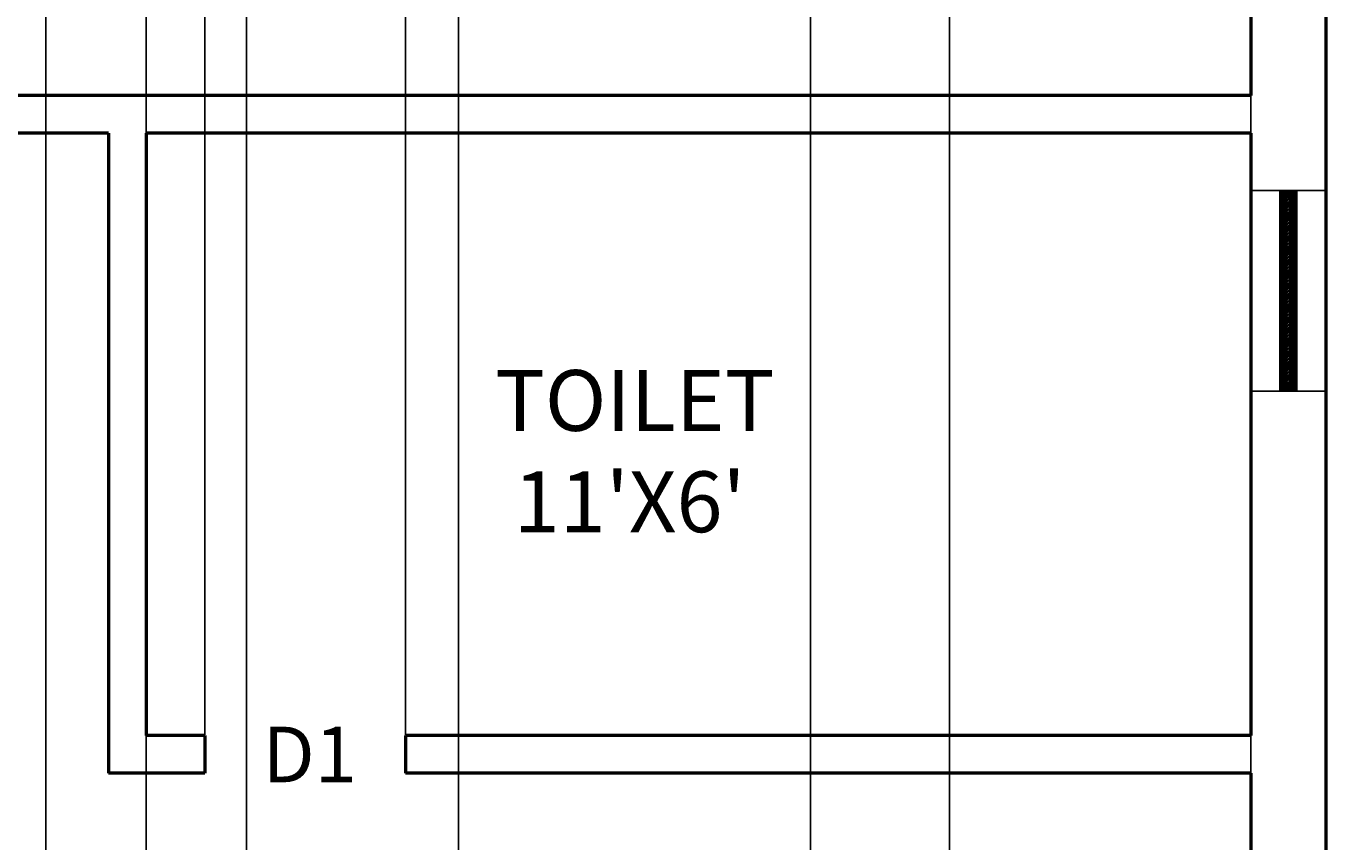
# Model space of a CAD drawing. Units: inches. Extents: x 338 to 1188, y -996 to 127.
# Tile 12 of 15: x 802 to 957, y -483 to -385. Entities that reach past the tile are written whole.
import ezdxf

# ---------------------------------------------------------------- set-up
doc = ezdxf.new("R2010")
doc.units = ezdxf.units.IN
doc.header["$MEASUREMENT"] = 0
for name, color, linetype, lineweight in [('A-ANNO-DIMS', 5, 'Continuous', 18), ('A-ANNO-TEXT', 7, 'Continuous', 18), ('A-AREA-IDEN', 8, 'Continuous', 18), ('A-GLAZ-PATT', 5, 'Continuous', 13), ('wall', 1, 'Continuous', 50), ('win', 5, 'Continuous', 25)]:
    doc.layers.add(name, color=color, linetype=linetype, lineweight=lineweight)
doc.styles.get("Standard").update_dxf_attribs({"font": 'arial.ttf'})
doc.dimstyles.get("Standard").update_dxf_attribs({"dimtxt": 0.18, "dimasz": 0.18, "dimexe": 0.18, "dimexo": 0.0625, "dimgap": 0.09, "dimtad": 0, "dimtih": 1, "dimtoh": 1, "dimdec": 1, "dimzin": 0, "dimdsep": 46, "dimlunit": 4, "dimtxsty": 'Standard', "dimcen": 0.09, "dimadec": 0, "dimazin": 0, "dimtfac": 1, "dimtdec": 1, "dimtofl": 0, "dimtmove": 0, "dimatfit": 3, "dimfxl": 1, "dimtolj": 1, "dimtzin": 0, "dimarcsym": 0})

# ---------------------------------------------------------------- blocks, each defined once
blk = doc.blocks.new('*D26')
at = {"layer": 'A-ANNO-DIMS', "color": 0, "lineweight": -2, "transparency": 16777216}
for p, q in [((815.96, -297.8), (815.96, -968.86)), ((827.96, -297.8), (827.96, -968.86)), ((816.14, -968.68), (821.64, -968.68)), ((827.78, -968.68), (822.28, -968.68))]:
    blk.add_line(p, q, dxfattribs=at)
at = {"layer": 'A-ANNO-DIMS', "color": 0, "transparency": 16777216}
for points in [[(816.14, -968.65), (816.14, -968.71), (815.96, -968.68)], [(827.78, -968.65), (827.78, -968.71), (827.96, -968.68)]]:
    blk.add_solid(points, dxfattribs=at)
at = {"layer": 'Defpoints', "color": 0, "transparency": 16777216}
for p in [(815.96, -297.73), (827.96, -297.73), (827.96, -968.68)]:
    blk.add_point(p, dxfattribs=at)
at = {"layer": 'A-ANNO-DIMS', "color": 0, "transparency": 16777216, "insert": (821.96, -968.68), "char_height": 0.18, "attachment_point": 5}
blk.add_mtext('\\A1;1\'-0"', dxfattribs=at)
blk = doc.blocks.new('*D27')
at = {"layer": 'A-ANNO-DIMS', "color": 0, "lineweight": -2, "transparency": 16777216}
for p, q in [((911.96, -297.8), (911.96, -968.86)), ((947.96, -297.8), (947.96, -968.86)), ((912.14, -968.68), (929.63, -968.68)), ((947.78, -968.68), (930.29, -968.68))]:
    blk.add_line(p, q, dxfattribs=at)
at = {"layer": 'A-ANNO-DIMS', "color": 0, "transparency": 16777216}
for points in [[(912.14, -968.65), (912.14, -968.71), (911.96, -968.68)], [(947.78, -968.65), (947.78, -968.71), (947.96, -968.68)]]:
    blk.add_solid(points, dxfattribs=at)
at = {"layer": 'Defpoints', "color": 0, "transparency": 16777216}
for p in [(911.96, -297.73), (947.96, -297.73), (947.96, -968.68)]:
    blk.add_point(p, dxfattribs=at)
at = {"layer": 'A-ANNO-DIMS', "color": 0, "transparency": 16777216, "insert": (929.96, -968.68), "char_height": 0.18, "attachment_point": 5}
blk.add_mtext('\\A1;3\'-0"', dxfattribs=at)
blk = doc.blocks.new('*D28')
at = {"layer": 'A-ANNO-DIMS', "color": 0, "lineweight": -2, "transparency": 16777216}
for p, q in [((803.96, -265.8), (803.96, -968.86)), ((947.96, -297.8), (947.96, -968.86)), ((804.14, -968.68), (875.57, -968.68)), ((947.78, -968.68), (876.35, -968.68))]:
    blk.add_line(p, q, dxfattribs=at)
at = {"layer": 'A-ANNO-DIMS', "color": 0, "transparency": 16777216}
for points in [[(804.14, -968.65), (804.14, -968.71), (803.96, -968.68)], [(947.78, -968.65), (947.78, -968.71), (947.96, -968.68)]]:
    blk.add_solid(points, dxfattribs=at)
at = {"layer": 'Defpoints', "color": 0, "transparency": 16777216}
for p in [(803.96, -265.73), (947.96, -297.73), (947.96, -968.68)]:
    blk.add_point(p, dxfattribs=at)
at = {"layer": 'A-ANNO-DIMS', "color": 0, "transparency": 16777216, "insert": (875.96, -968.68), "char_height": 0.18, "attachment_point": 5}
blk.add_mtext('\\A1;12\'-0"', dxfattribs=at)
blk = doc.blocks.new('*D38')
at = {"layer": 'A-ANNO-DIMS', "color": 0, "lineweight": -2, "transparency": 16777216}
for p, q in [((822.96, -470.17), (822.96, 67.25)), ((823.14, 67.07), (834.63, 67.07)), ((846.78, 67.07), (835.29, 67.07)), ((846.96, -470.17), (846.96, 67.25))]:
    blk.add_line(p, q, dxfattribs=at)
at = {"layer": 'A-ANNO-DIMS', "color": 0, "transparency": 16777216}
for points in [[(823.14, 67.1), (823.14, 67.04), (822.96, 67.07)], [(846.78, 67.1), (846.78, 67.04), (846.96, 67.07)]]:
    blk.add_solid(points, dxfattribs=at)
at = {"layer": 'Defpoints', "color": 0, "transparency": 16777216}
for p in [(846.96, 67.07), (822.96, -470.23), (846.96, -470.23)]:
    blk.add_point(p, dxfattribs=at)
at = {"layer": 'A-ANNO-DIMS', "color": 0, "transparency": 16777216, "insert": (834.96, 67.07), "char_height": 0.18, "attachment_point": 5}
blk.add_mtext('\\A1;2\'-0"', dxfattribs=at)
blk = doc.blocks.new('*D43')
at = {"layer": 'A-ANNO-DIMS', "color": 0, "lineweight": -2, "transparency": 16777216}
for p, q in [((853.28, -53.93), (853.28, -968.86)), ((895.37, -53.93), (895.37, -968.86)), ((853.46, -968.68), (873.99, -968.68)), ((895.19, -968.68), (874.65, -968.68))]:
    blk.add_line(p, q, dxfattribs=at)
at = {"layer": 'A-ANNO-DIMS', "color": 0, "transparency": 16777216}
for points in [[(853.46, -968.65), (853.46, -968.71), (853.28, -968.68)], [(895.19, -968.65), (895.19, -968.71), (895.37, -968.68)]]:
    blk.add_solid(points, dxfattribs=at)
at = {"layer": 'Defpoints', "color": 0, "transparency": 16777216}
for p in [(853.28, -53.87), (895.37, -53.87), (895.37, -968.68)]:
    blk.add_point(p, dxfattribs=at)
at = {"layer": 'A-ANNO-DIMS', "color": 0, "transparency": 16777216, "insert": (874.32, -968.68), "char_height": 0.18, "attachment_point": 5}
blk.add_mtext('\\A1;3\'-6"', dxfattribs=at)
blk = doc.blocks.new('*D44')
at = {"layer": 'A-ANNO-DIMS', "color": 0, "lineweight": -2, "transparency": 16777216}
for p, q in [((895.37, -53.93), (895.37, -968.86)), ((947.96, -54.8), (947.96, -968.86)), ((895.55, -968.68), (921.12, -968.68)), ((947.78, -968.68), (922.21, -968.68))]:
    blk.add_line(p, q, dxfattribs=at)
at = {"layer": 'A-ANNO-DIMS', "color": 0, "transparency": 16777216}
for points in [[(895.55, -968.65), (895.55, -968.71), (895.37, -968.68)], [(947.78, -968.65), (947.78, -968.71), (947.96, -968.68)]]:
    blk.add_solid(points, dxfattribs=at)
at = {"layer": 'Defpoints', "color": 0, "transparency": 16777216}
for p in [(895.37, -53.87), (947.96, -54.73), (947.96, -968.68)]:
    blk.add_point(p, dxfattribs=at)
at = {"layer": 'A-ANNO-DIMS', "color": 0, "transparency": 16777216, "insert": (921.67, -968.68), "char_height": 0.18, "attachment_point": 5}
blk.add_mtext('\\A1;4\'-4 1/2"', dxfattribs=at)
blk = doc.blocks.new('*D47')
at = {"layer": 'A-ANNO-DIMS', "color": 0, "lineweight": -2, "transparency": 16777216}
for p, q in [((759.67, -755.17), (759.67, 67.25)), ((759.85, 67.07), (867.68, 67.07)), ((976.28, 67.07), (868.46, 67.07)), ((976.46, -755.17), (976.46, 67.25))]:
    blk.add_line(p, q, dxfattribs=at)
at = {"layer": 'A-ANNO-DIMS', "color": 0, "transparency": 16777216}
for points in [[(759.85, 67.1), (759.85, 67.04), (759.67, 67.07)], [(976.28, 67.1), (976.28, 67.04), (976.46, 67.07)]]:
    blk.add_solid(points, dxfattribs=at)
at = {"layer": 'Defpoints', "color": 0, "transparency": 16777216}
for p in [(976.46, 67.07), (759.67, -755.23), (976.46, -755.23)]:
    blk.add_point(p, dxfattribs=at)
at = {"layer": 'A-ANNO-DIMS', "color": 0, "transparency": 16777216, "insert": (868.07, 67.07), "char_height": 0.18, "attachment_point": 5}
blk.add_mtext('\\A1;18\'-1"', dxfattribs=at)

msp = doc.modelspace()

# ---------------------------------------------------------------- hatches: boundary and pattern name
at = {"layer": 'A-GLAZ-PATT'}
h = msp.add_hatch(dxfattribs=at)
h.set_pattern_fill('ANSI31', color=256)
h.paths.add_polyline_path([(953.46, -405.07), (951.46, -405.07), (951.46, -429.07), (953.46, -429.07)])
h.paths.add_polyline_path([(953.46, -485.22), (951.46, -485.22), (951.46, -521.22), (953.46, -521.22)])
h.paths.add_polyline_path([(794.21, -19.23), (758.21, -19.23), (758.21, -21.23), (794.21, -21.23)])
h.paths.add_polyline_path([(668.69, -19.23), (632.69, -19.23), (632.69, -21.23), (668.69, -21.23)])
h.paths.add_polyline_path([(602.46, -94.89), (600.46, -94.89), (600.46, -130.89), (602.46, -130.89)])
h.paths.add_polyline_path([(602.46, -243.73), (600.46, -243.73), (600.46, -315.73), (602.46, -315.73)])

# ---------------------------------------------------------------- linework, layer by layer
at = {"layer": 'wall'}
for p, q in [((956.96, -15.73), (956.96, -615.73)), ((947.96, -149.23), (947.96, -393.73)), ((947.96, -393.73), (788.96, -393.73)), ((811.46, -398.23), (788.96, -398.23)), ((811.46, -398.23), (811.46, -474.73)), ((815.96, -398.23), (815.96, -470.23)), ((947.96, -398.23), (815.96, -398.23)), ((947.96, -398.23), (947.96, -470.23)), ((822.96, -470.23), (815.96, -470.23)), ((822.96, -470.23), (822.96, -474.73)), ((947.96, -470.23), (846.96, -470.23)), ((846.96, -470.23), (846.96, -474.73)), ((822.96, -474.73), (811.46, -474.73)), ((947.96, -474.73), (846.96, -474.73)), ((947.96, -474.73), (947.96, -606.73))]:
    msp.add_line(p, q, dxfattribs=at)
at = {"layer": 'win'}
for p, q in [((947.96, -405.07), (956.96, -405.07)), ((951.46, -405.07), (951.46, -429.07)), ((953.46, -405.07), (953.46, -429.07)), ((947.96, -429.07), (956.96, -429.07))]:
    msp.add_line(p, q, dxfattribs=at)

# ---------------------------------------------------------------- texts
at = {"layer": 'A-ANNO-TEXT'}
msp.add_text('D1', height=6.652, dxfattribs=at).set_placement((829.86, -475.84))
at = {"layer": 'A-AREA-IDEN', "insert": (851, -426.55), "char_height": 7.27, "attachment_point": 1}
msp.add_mtext_dynamic_manual_height_columns("   TOILET\\P    11'X6'", width=54.3765, gutter_width=1, heights=[0], dxfattribs=at)

# ---------------------------------------------------------------- dimensions: what is measured, and where the dimension line sits
at = {"layer": 'A-ANNO-DIMS'}
for base, p1, p2, picture, middle in [((976.46, 67.07), (759.67, -755.23), (976.46, -755.23), '*D47', (868.07, 67.07)), ((846.96, 67.07), (822.96, -470.23), (846.96, -470.23), '*D38', (834.96, 67.07)), ((895.37, -968.68), (853.28, -53.87), (895.37, -53.87), '*D43', (874.32, -968.68)), ((947.96, -968.68), (895.37, -53.87), (947.96, -54.73), '*D44', (921.67, -968.68)), ((947.96, -968.68), (803.96, -265.73), (947.96, -297.73), '*D28', (875.96, -968.68)), ((827.96, -968.68), (815.96, -297.73), (827.96, -297.73), '*D26', (821.96, -968.68)), ((947.96, -968.68), (911.96, -297.73), (947.96, -297.73), '*D27', (929.96, -968.68))]:
    dim = msp.add_linear_dim(base=base, p1=p1, p2=p2, dimstyle='Standard', override={"dimdec": 1, "dimlfac": 1, "dimrnd": 0, "dimzin": 1, "dimdsep": 46, "dimlunit": 4, "dimfrac": 2}, dxfattribs=at)
    dim.commit()
    dim.dimension.update_dxf_attribs({"geometry": picture, "text_midpoint": middle})

doc.saveas('drawing.dxf')
